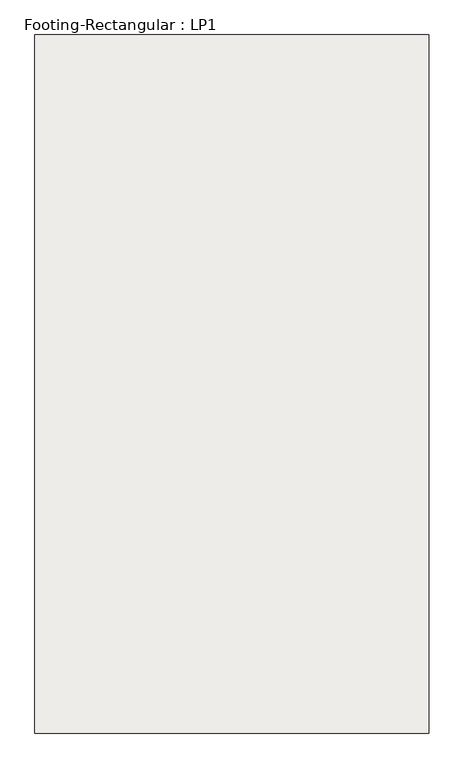
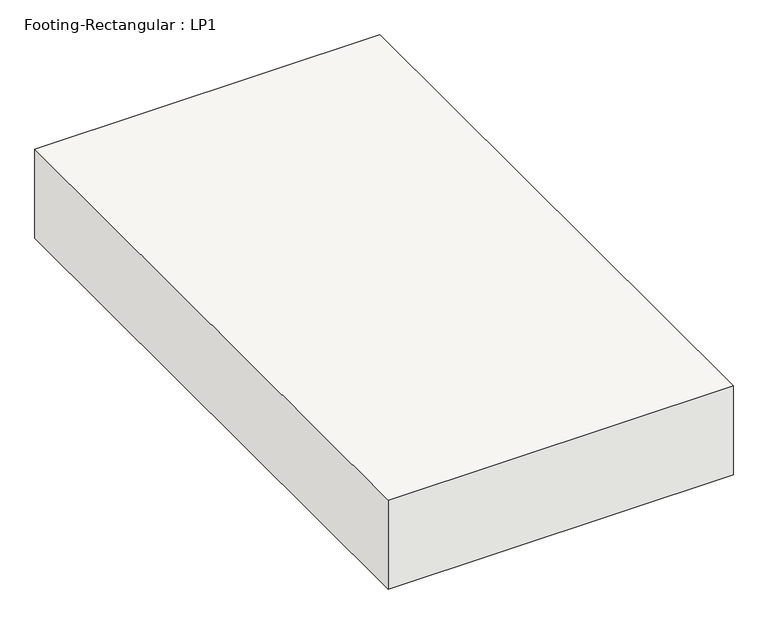
"""IFC4 building model written with IfcOpenShell, lengths in millimetres: slab geometry, Footing-Rectangular : LP1."""

from ifc_helpers import new_model, si_unit, frame, origin, place, context, project, spatial, polyline, outline, extrude, source, transform, mapped, element, save


def footing_rectangular_lp1_8d3386b4(model_context):
    return source(origin(), model_context, "Body", "SweptSolid", [
        extrude(outline(polyline([(838.2, 1485.9), (838.2, -1485.9), (-838.2, -1485.9), (-838.2, 1485.9), (838.2, 1485.9)])), frame((0.0, 0.0, -457.2), z_axis=(0.0, 0.0, 1.0), x_axis=(1.0, 0.0, 0.0)), (0.0, 0.0, 1.0), 457.2),
    ])


if __name__ == "__main__":
    model = new_model("IFC4")
    model_context = context("Model", 3, world=origin())
    ifc_project = project(units=[si_unit("LENGTHUNIT", "METRE", prefix="MILLI")], contexts=[model_context])
    site = spatial("IfcSite", under=ifc_project)
    building = spatial("IfcBuilding", under=site)
    placement = place(None, origin())
    footing_rectangular_lp1_shape = footing_rectangular_lp1_8d3386b4(model_context)
    element("IfcSlab", 1, ObjectType="Footing-Rectangular : LP1", at=placement, inside=building, context=model_context, shape_type="MappedRepresentation", body=[
        mapped(footing_rectangular_lp1_shape, transform((0.0, 0.0, 0.0), x_axis=(1.0, 0.0, 0.0), y_axis=(0.0, 1.0, 0.0), z_axis=(0.0, 0.0, 1.0))),
    ])
    save(model, "model.ifc")

# Revit data of these elements
# Type "Footing-Rectangular : LP1"
#   Width = 1676.4 mm
#   Length = 2971.8 mm
#   Foundation Thickness = 457.2 mm
#   Structural Material [instance default] = Concrete - Cast-in-Place Concrete
#   Assembly Code = ""
# Element 1 (IfcSlab, "Footing-Rectangular : LP1")
#   Materials on its faces: "Concrete - Cast-in-Place Concrete"
# Materials
#   "Concrete - Cast-in-Place Concrete": class "Concrete", colour RGB 192 192 192, transparency 0, Cost = 0
